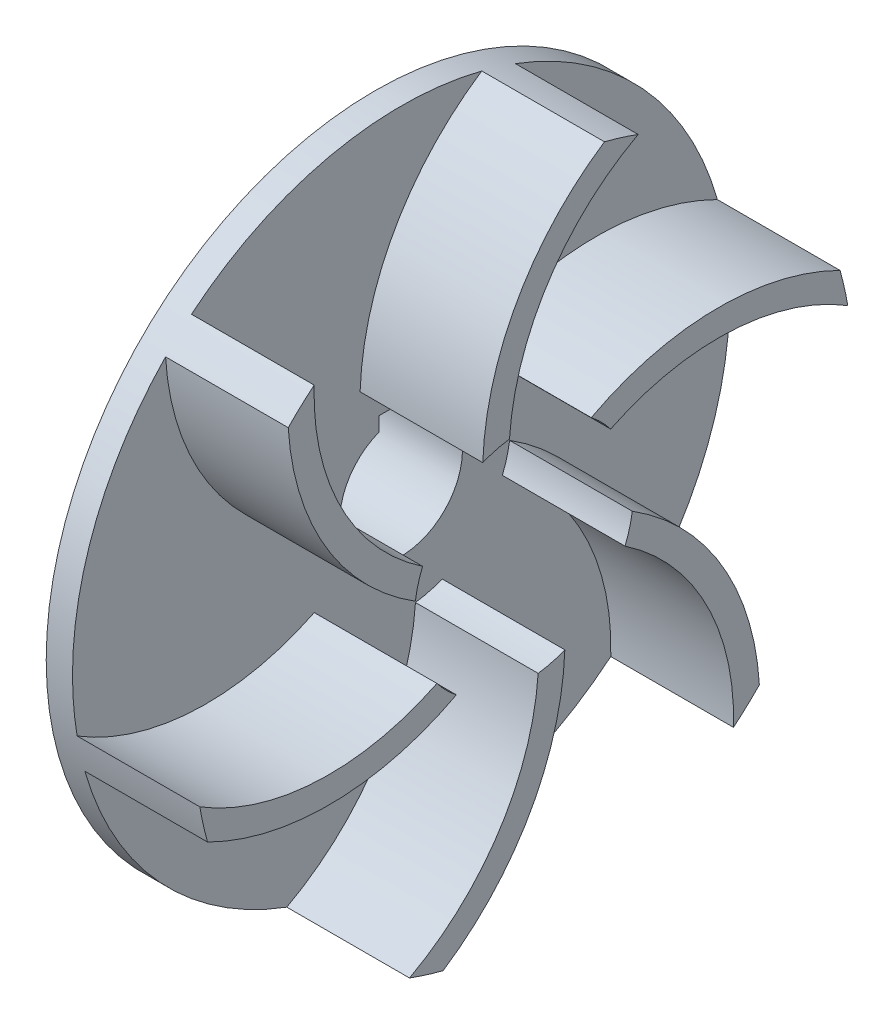
ISO-10303-21;
HEADER;
FILE_DESCRIPTION(('STEP AP214'),'2;1');
FILE_NAME('part.step','',(''),(''),'','','');
FILE_SCHEMA(('AUTOMOTIVE_DESIGN { 1 0 10303 214 1 1 1 1 }'));
ENDSEC;
DATA;
#1=APPLICATION_CONTEXT('core data for automotive mechanical design processes');
#2=APPLICATION_PROTOCOL_DEFINITION('international standard','automotive_design',2000,#1);
#3=PRODUCT_CONTEXT('',#1,'mechanical');
#4=PRODUCT('Part','Part','',(#3));
#5=PRODUCT_RELATED_PRODUCT_CATEGORY('part','',(#4));
#6=PRODUCT_DEFINITION_FORMATION('','',#4);
#7=PRODUCT_DEFINITION_CONTEXT('part definition',#1,'design');
#8=PRODUCT_DEFINITION('design','',#6,#7);
#9=PRODUCT_DEFINITION_SHAPE('','',#8);
#10=(LENGTH_UNIT() NAMED_UNIT(*) SI_UNIT(.MILLI.,.METRE.));
#11=(NAMED_UNIT(*) PLANE_ANGLE_UNIT() SI_UNIT($,.RADIAN.));
#12=(NAMED_UNIT(*) SI_UNIT($,.STERADIAN.) SOLID_ANGLE_UNIT());
#13=UNCERTAINTY_MEASURE_WITH_UNIT(LENGTH_MEASURE(1.E-05),#10,'distance_accuracy_value','');
#14=(GEOMETRIC_REPRESENTATION_CONTEXT(3) GLOBAL_UNCERTAINTY_ASSIGNED_CONTEXT((#13)) GLOBAL_UNIT_ASSIGNED_CONTEXT((#10,
#11,#12)) REPRESENTATION_CONTEXT('',''));
#15=CARTESIAN_POINT('',(0.,0.,0.));
#16=DIRECTION('',(0.,0.,1.));
#17=DIRECTION('',(1.,0.,0.));
#18=AXIS2_PLACEMENT_3D('',#15,#16,#17);
#19=CARTESIAN_POINT('',(19.,37.5,0.));
#20=DIRECTION('',(-1.,0.,0.));
#21=DIRECTION('',(0.,0.,1.));
#22=AXIS2_PLACEMENT_3D('',#19,#20,#21);
#23=PLANE('',#22);
#24=CARTESIAN_POINT('',(19.,-17.5291013565556,-22.2360825665268));
#25=DIRECTION('',(1.,0.,0.));
#26=DIRECTION('',(0.,0.,-1.));
#27=AXIS2_PLACEMENT_3D('',#24,#25,#26);
#28=CIRCLE('',#27,31.);
#29=CARTESIAN_POINT('',(19.,10.2057241564115,-36.0845284636399));
#30=VERTEX_POINT('',#29);
#31=CARTESIAN_POINT('',(19.,9.84966379316857,-7.69637077859064));
#32=VERTEX_POINT('',#31);
#33=EDGE_CURVE('E290',#30,#32,#28,.T.);
#34=ORIENTED_EDGE('',*,*,#33,.F.);
#35=CARTESIAN_POINT('',(19.,0.,0.));
#36=DIRECTION('',(-1.,0.,0.));
#37=DIRECTION('',(0.,0.,1.));
#38=AXIS2_PLACEMENT_3D('',#35,#36,#37);
#39=CIRCLE('',#38,37.5);
#40=CARTESIAN_POINT('',(19.,35.1575351750676,-13.0459848387879));
#41=VERTEX_POINT('',#40);
#42=EDGE_CURVE('E847',#41,#30,#39,.T.);
#43=ORIENTED_EDGE('',*,*,#42,.F.);
#44=CARTESIAN_POINT('',(19.,10.4924617049827,-26.2986883635528));
#45=DIRECTION('',(1.,0.,0.));
#46=DIRECTION('',(0.,0.,-1.));
#47=AXIS2_PLACEMENT_3D('',#44,#45,#46);
#48=CIRCLE('',#47,28.);
#49=CARTESIAN_POINT('',(19.,12.3923748695187,1.63677887734412));
#50=VERTEX_POINT('',#49);
#51=EDGE_CURVE('E346',#41,#50,#48,.T.);
#52=ORIENTED_EDGE('',*,*,#51,.T.);
#53=CARTESIAN_POINT('',(19.,0.,0.));
#54=DIRECTION('',(1.,0.,0.));
#55=DIRECTION('',(0.,0.,-1.));
#56=AXIS2_PLACEMENT_3D('',#53,#54,#55);
#57=CIRCLE('',#56,12.5);
#58=CARTESIAN_POINT('',(19.,11.590084507788,4.68187367432452));
#59=VERTEX_POINT('',#58);
#60=EDGE_CURVE('E354',#50,#59,#57,.T.);
#61=ORIENTED_EDGE('',*,*,#60,.T.);
#62=CARTESIAN_POINT('',(19.,10.4924617049827,-26.2986883635528));
#63=DIRECTION('',(1.,0.,0.));
#64=DIRECTION('',(0.,0.,-1.));
#65=AXIS2_PLACEMENT_3D('',#62,#63,#64);
#66=CIRCLE('',#65,31.);
#67=CARTESIAN_POINT('',(19.,36.3529804113006,-9.20384784835101));
#68=VERTEX_POINT('',#67);
#69=EDGE_CURVE('E345',#68,#59,#66,.T.);
#70=ORIENTED_EDGE('',*,*,#69,.F.);
#71=CARTESIAN_POINT('',(19.,28.8769218753108,23.9243261766596));
#72=VERTEX_POINT('',#71);
#73=EDGE_CURVE('E479',#72,#68,#39,.T.);
#74=ORIENTED_EDGE('',*,*,#73,.F.);
#75=CARTESIAN_POINT('',(19.,28.0215630615383,-4.06260579702601));
#76=DIRECTION('',(1.,0.,0.));
#77=DIRECTION('',(0.,0.,-1.));
#78=AXIS2_PLACEMENT_3D('',#75,#76,#77);
#79=CIRCLE('',#78,28.0000000000001);
#80=CARTESIAN_POINT('',(19.,4.77869534660156,11.5505008888952));
#81=VERTEX_POINT('',#80);
#82=EDGE_CURVE('E115',#72,#81,#79,.T.);
#83=ORIENTED_EDGE('',*,*,#82,.T.);
#84=CARTESIAN_POINT('',(19.,0.,0.));
#85=DIRECTION('',(1.,0.,0.));
#86=DIRECTION('',(0.,0.,-1.));
#87=AXIS2_PLACEMENT_3D('',#84,#85,#86);
#88=CIRCLE('',#87,12.5);
#89=CARTESIAN_POINT('',(19.,1.74042071461927,12.3782444529151));
#90=VERTEX_POINT('',#89);
#91=EDGE_CURVE('E318',#81,#90,#88,.T.);
#92=ORIENTED_EDGE('',*,*,#91,.T.);
#93=CARTESIAN_POINT('',(19.,28.0215630615383,-4.06260579702601));
#94=DIRECTION('',(1.,0.,0.));
#95=DIRECTION('',(0.,0.,-1.));
#96=AXIS2_PLACEMENT_3D('',#93,#94,#95);
#97=CIRCLE('',#96,31.0000000000001);
#98=CARTESIAN_POINT('',(19.,26.147256254889,26.8806806152889));
#99=VERTEX_POINT('',#98);
#100=EDGE_CURVE('E325',#99,#90,#97,.T.);
#101=ORIENTED_EDGE('',*,*,#100,.F.);
#102=CARTESIAN_POINT('',(19.,-6.28061329975611,36.9703110154476));
#103=VERTEX_POINT('',#102);
#104=EDGE_CURVE('E474',#103,#99,#39,.T.);
#105=ORIENTED_EDGE('',*,*,#104,.F.);
#106=CARTESIAN_POINT('',(19.,17.5291013565557,22.2360825665265));
#107=DIRECTION('',(1.,0.,0.));
#108=DIRECTION('',(0.,0.,-1.));
#109=AXIS2_PLACEMENT_3D('',#106,#107,#108);
#110=CIRCLE('',#109,27.9999999999998);
#111=CARTESIAN_POINT('',(19.,-7.61367952291693,9.91372201155118));
#112=VERTEX_POINT('',#111);
#113=EDGE_CURVE('E436',#103,#112,#110,.T.);
#114=ORIENTED_EDGE('',*,*,#113,.T.);
#115=CARTESIAN_POINT('',(19.,0.,0.));
#116=DIRECTION('',(1.,0.,0.));
#117=DIRECTION('',(0.,0.,-1.));
#118=AXIS2_PLACEMENT_3D('',#115,#116,#117);
#119=CIRCLE('',#118,12.5);
#120=CARTESIAN_POINT('',(19.,-9.84966379316844,7.69637077859072));
#121=VERTEX_POINT('',#120);
#122=EDGE_CURVE('E414',#112,#121,#119,.T.);
#123=ORIENTED_EDGE('',*,*,#122,.T.);
#124=CARTESIAN_POINT('',(19.,17.5291013565557,22.2360825665265));
#125=DIRECTION('',(1.,0.,0.));
#126=DIRECTION('',(0.,0.,-1.));
#127=AXIS2_PLACEMENT_3D('',#124,#125,#126);
#128=CIRCLE('',#127,30.9999999999998);
#129=CARTESIAN_POINT('',(19.,-10.2057241564109,36.0845284636401));
#130=VERTEX_POINT('',#129);
#131=EDGE_CURVE('E426',#130,#121,#128,.T.);
#132=ORIENTED_EDGE('',*,*,#131,.F.);
#133=CARTESIAN_POINT('',(19.,-35.1575351750675,13.0459848387883));
#134=VERTEX_POINT('',#133);
#135=EDGE_CURVE('E475',#134,#130,#39,.T.);
#136=ORIENTED_EDGE('',*,*,#135,.F.);
#137=CARTESIAN_POINT('',(19.,-10.4924617049824,26.2986883635528));
#138=DIRECTION('',(1.,0.,0.));
#139=DIRECTION('',(0.,0.,-1.));
#140=AXIS2_PLACEMENT_3D('',#137,#138,#139);
#141=CIRCLE('',#140,28.);
#142=CARTESIAN_POINT('',(19.,-12.3923748695188,-1.6367788773441));
#143=VERTEX_POINT('',#142);
#144=EDGE_CURVE('E408',#134,#143,#141,.T.);
#145=ORIENTED_EDGE('',*,*,#144,.T.);
#146=CARTESIAN_POINT('',(19.,0.,0.));
#147=DIRECTION('',(1.,0.,0.));
#148=DIRECTION('',(0.,0.,-1.));
#149=AXIS2_PLACEMENT_3D('',#146,#147,#148);
#150=CIRCLE('',#149,12.5);
#151=CARTESIAN_POINT('',(19.,-11.590084507788,-4.6818736743245));
#152=VERTEX_POINT('',#151);
#153=EDGE_CURVE('E406',#143,#152,#150,.T.);
#154=ORIENTED_EDGE('',*,*,#153,.T.);
#155=CARTESIAN_POINT('',(19.,-10.4924617049824,26.2986883635528));
#156=DIRECTION('',(1.,0.,0.));
#157=DIRECTION('',(0.,0.,-1.));
#158=AXIS2_PLACEMENT_3D('',#155,#156,#157);
#159=CIRCLE('',#158,31.);
#160=CARTESIAN_POINT('',(19.,-36.3529804113005,9.20384784835134));
#161=VERTEX_POINT('',#160);
#162=EDGE_CURVE('E401',#161,#152,#159,.T.);
#163=ORIENTED_EDGE('',*,*,#162,.F.);
#164=CARTESIAN_POINT('',(19.,-28.8769218753109,-23.9243261766594));
#165=VERTEX_POINT('',#164);
#166=EDGE_CURVE('E851',#165,#161,#39,.T.);
#167=ORIENTED_EDGE('',*,*,#166,.F.);
#168=CARTESIAN_POINT('',(19.,-28.0215630615381,4.06260579702616));
#169=DIRECTION('',(1.,0.,0.));
#170=DIRECTION('',(0.,0.,-1.));
#171=AXIS2_PLACEMENT_3D('',#168,#169,#170);
#172=CIRCLE('',#171,28.);
#173=CARTESIAN_POINT('',(19.,-4.77869534660156,-11.5505008888952));
#174=VERTEX_POINT('',#173);
#175=EDGE_CURVE('E380',#165,#174,#172,.T.);
#176=ORIENTED_EDGE('',*,*,#175,.T.);
#177=CARTESIAN_POINT('',(19.,0.,0.));
#178=DIRECTION('',(1.,0.,0.));
#179=DIRECTION('',(0.,0.,-1.));
#180=AXIS2_PLACEMENT_3D('',#177,#178,#179);
#181=CIRCLE('',#180,12.5);
#182=CARTESIAN_POINT('',(19.,-1.7404207146193,-12.3782444529152));
#183=VERTEX_POINT('',#182);
#184=EDGE_CURVE('E381',#174,#183,#181,.T.);
#185=ORIENTED_EDGE('',*,*,#184,.T.);
#186=CARTESIAN_POINT('',(19.,-28.0215630615381,4.06260579702616));
#187=DIRECTION('',(1.,0.,0.));
#188=DIRECTION('',(0.,0.,-1.));
#189=AXIS2_PLACEMENT_3D('',#186,#187,#188);
#190=CIRCLE('',#189,31.0000000000001);
#191=CARTESIAN_POINT('',(19.,-26.1472562548891,-26.8806806152888));
#192=VERTEX_POINT('',#191);
#193=EDGE_CURVE('E372',#192,#183,#190,.T.);
#194=ORIENTED_EDGE('',*,*,#193,.F.);
#195=CARTESIAN_POINT('',(19.,6.28061329975673,-36.9703110154475));
#196=VERTEX_POINT('',#195);
#197=EDGE_CURVE('E293',#196,#192,#39,.T.);
#198=ORIENTED_EDGE('',*,*,#197,.F.);
#199=CARTESIAN_POINT('',(19.,-17.5291013565556,-22.2360825665268));
#200=DIRECTION('',(1.,0.,0.));
#201=DIRECTION('',(0.,0.,-1.));
#202=AXIS2_PLACEMENT_3D('',#199,#200,#201);
#203=CIRCLE('',#202,28.);
#204=CARTESIAN_POINT('',(19.,7.61367952291712,-9.91372201155109));
#205=VERTEX_POINT('',#204);
#206=EDGE_CURVE('E102',#196,#205,#203,.T.);
#207=ORIENTED_EDGE('',*,*,#206,.T.);
#208=CARTESIAN_POINT('',(19.,0.,0.));
#209=DIRECTION('',(1.,0.,0.));
#210=DIRECTION('',(0.,0.,-1.));
#211=AXIS2_PLACEMENT_3D('',#208,#209,#210);
#212=CIRCLE('',#211,12.5);
#213=EDGE_CURVE('E285',#205,#32,#212,.T.);
#214=ORIENTED_EDGE('',*,*,#213,.T.);
#215=EDGE_LOOP('',(#34,#43,#52,#61,#70,#74,#83,#92,#101,#105,#114,#123,#132,#136,#145,#154,#163,
#167,#176,#185,#194,#198,#207,#214));
#216=FACE_BOUND('',#215,.T.);
#217=CARTESIAN_POINT('',(19.,0.,0.));
#218=DIRECTION('',(-1.,0.,0.));
#219=DIRECTION('',(0.,0.,1.));
#220=AXIS2_PLACEMENT_3D('',#217,#218,#219);
#221=CIRCLE('',#220,7.);
#222=CARTESIAN_POINT('',(19.,6.53834841531101,-2.5));
#223=VERTEX_POINT('',#222);
#224=CARTESIAN_POINT('',(19.,6.53834841531101,2.5));
#225=VERTEX_POINT('',#224);
#226=EDGE_CURVE('E476',#223,#225,#221,.T.);
#227=ORIENTED_EDGE('',*,*,#226,.T.);
#228=DIRECTION('',(0.,1.,0.));
#229=VECTOR('',#228,1.);
#230=CARTESIAN_POINT('',(19.,37.5,2.5));
#231=LINE('',#230,#229);
#232=CARTESIAN_POINT('',(19.,8.15,2.5));
#233=VERTEX_POINT('',#232);
#234=EDGE_CURVE('E12',#225,#233,#231,.T.);
#235=ORIENTED_EDGE('',*,*,#234,.T.);
#236=DIRECTION('',(0.,0.,-1.));
#237=VECTOR('',#236,1.);
#238=CARTESIAN_POINT('',(19.,8.15,0.));
#239=LINE('',#238,#237);
#240=CARTESIAN_POINT('',(19.,8.15,-2.5));
#241=VERTEX_POINT('',#240);
#242=EDGE_CURVE('E488',#233,#241,#239,.T.);
#243=ORIENTED_EDGE('',*,*,#242,.T.);
#244=DIRECTION('',(0.,-1.,0.));
#245=VECTOR('',#244,1.);
#246=CARTESIAN_POINT('',(19.,37.5,-2.5));
#247=LINE('',#246,#245);
#248=EDGE_CURVE('E100',#241,#223,#247,.T.);
#249=ORIENTED_EDGE('',*,*,#248,.T.);
#250=EDGE_LOOP('',(#227,#235,#243,#249));
#251=FACE_BOUND('',#250,.T.);
#252=ADVANCED_FACE('F90',(#216,#251),#23,.F.);
#253=CARTESIAN_POINT('',(-28.,0.,0.));
#254=DIRECTION('',(-1.,0.,0.));
#255=DIRECTION('',(0.,0.,1.));
#256=AXIS2_PLACEMENT_3D('',#253,#254,#255);
#257=CYLINDRICAL_SURFACE('',#256,12.5);
#258=CARTESIAN_POINT('',(0.,0.,0.));
#259=DIRECTION('',(-1.,0.,0.));
#260=DIRECTION('',(0.,0.,1.));
#261=AXIS2_PLACEMENT_3D('',#258,#259,#260);
#262=CIRCLE('',#261,12.5);
#263=CARTESIAN_POINT('',(0.,0.,12.5));
#264=VERTEX_POINT('',#263);
#265=EDGE_CURVE('E484',#264,#264,#262,.T.);
#266=ORIENTED_EDGE('',*,*,#265,.F.);
#267=EDGE_LOOP('',(#266));
#268=FACE_BOUND('',#267,.T.);
#269=CARTESIAN_POINT('',(16.,0.,0.));
#270=DIRECTION('',(-1.,0.,0.));
#271=DIRECTION('',(0.,0.,1.));
#272=AXIS2_PLACEMENT_3D('',#269,#270,#271);
#273=CIRCLE('',#272,12.5);
#274=CARTESIAN_POINT('',(16.,0.,12.5));
#275=VERTEX_POINT('',#274);
#276=EDGE_CURVE('E469',#275,#275,#273,.T.);
#277=ORIENTED_EDGE('',*,*,#276,.T.);
#278=EDGE_LOOP('',(#277));
#279=FACE_BOUND('',#278,.T.);
#280=ADVANCED_FACE('F93',(#268,#279),#257,.T.);
#281=CARTESIAN_POINT('',(0.,12.5,0.));
#282=DIRECTION('',(1.,0.,0.));
#283=DIRECTION('',(0.,0.,-1.));
#284=AXIS2_PLACEMENT_3D('',#281,#282,#283);
#285=PLANE('',#284);
#286=DIRECTION('',(0.,0.,-1.));
#287=VECTOR('',#286,1.);
#288=CARTESIAN_POINT('',(0.,8.15,-2.5));
#289=LINE('',#288,#287);
#290=CARTESIAN_POINT('',(0.,8.15,2.5));
#291=VERTEX_POINT('',#290);
#292=CARTESIAN_POINT('',(0.,8.15,-2.5));
#293=VERTEX_POINT('',#292);
#294=EDGE_CURVE('E452',#291,#293,#289,.T.);
#295=ORIENTED_EDGE('',*,*,#294,.F.);
#296=DIRECTION('',(0.,1.,0.));
#297=VECTOR('',#296,1.);
#298=CARTESIAN_POINT('',(0.,8.15,2.5));
#299=LINE('',#298,#297);
#300=CARTESIAN_POINT('',(0.,6.53834841531101,2.5));
#301=VERTEX_POINT('',#300);
#302=EDGE_CURVE('E446',#301,#291,#299,.T.);
#303=ORIENTED_EDGE('',*,*,#302,.F.);
#304=CARTESIAN_POINT('',(0.,0.,0.));
#305=DIRECTION('',(-1.,0.,0.));
#306=DIRECTION('',(0.,0.,1.));
#307=AXIS2_PLACEMENT_3D('',#304,#305,#306);
#308=CIRCLE('',#307,7.);
#309=CARTESIAN_POINT('',(0.,6.53834841531101,-2.5));
#310=VERTEX_POINT('',#309);
#311=EDGE_CURVE('E485',#310,#301,#308,.T.);
#312=ORIENTED_EDGE('',*,*,#311,.F.);
#313=DIRECTION('',(0.,-1.,0.));
#314=VECTOR('',#313,1.);
#315=CARTESIAN_POINT('',(0.,8.15,-2.5));
#316=LINE('',#315,#314);
#317=EDGE_CURVE('E455',#293,#310,#316,.T.);
#318=ORIENTED_EDGE('',*,*,#317,.F.);
#319=EDGE_LOOP('',(#295,#303,#312,#318));
#320=FACE_BOUND('',#319,.T.);
#321=ORIENTED_EDGE('',*,*,#265,.T.);
#322=EDGE_LOOP('',(#321));
#323=FACE_BOUND('',#322,.T.);
#324=ADVANCED_FACE('F502',(#320,#323),#285,.F.);
#325=CARTESIAN_POINT('',(-28.,0.,0.));
#326=DIRECTION('',(-1.,0.,0.));
#327=DIRECTION('',(0.,0.,1.));
#328=AXIS2_PLACEMENT_3D('',#325,#326,#327);
#329=CYLINDRICAL_SURFACE('',#328,7.);
#330=ORIENTED_EDGE('',*,*,#311,.T.);
#331=DIRECTION('',(-1.,0.,0.));
#332=VECTOR('',#331,1.);
#333=CARTESIAN_POINT('',(-28.,6.53834841531101,2.5));
#334=LINE('',#333,#332);
#335=EDGE_CURVE('E461',#301,#225,#334,.F.);
#336=ORIENTED_EDGE('',*,*,#335,.T.);
#337=ORIENTED_EDGE('',*,*,#226,.F.);
#338=DIRECTION('',(-1.,0.,0.));
#339=VECTOR('',#338,1.);
#340=CARTESIAN_POINT('',(-28.,6.53834841531101,-2.5));
#341=LINE('',#340,#339);
#342=EDGE_CURVE('E458',#223,#310,#341,.T.);
#343=ORIENTED_EDGE('',*,*,#342,.T.);
#344=EDGE_LOOP('',(#330,#336,#337,#343));
#345=FACE_BOUND('',#344,.T.);
#346=ADVANCED_FACE('F494',(#345),#329,.F.);
#347=CARTESIAN_POINT('',(-28.,0.,0.));
#348=DIRECTION('',(-1.,0.,0.));
#349=DIRECTION('',(0.,0.,1.));
#350=AXIS2_PLACEMENT_3D('',#347,#348,#349);
#351=CYLINDRICAL_SURFACE('',#350,37.5);
#352=CARTESIAN_POINT('',(16.,0.,0.));
#353=DIRECTION('',(-1.,0.,0.));
#354=DIRECTION('',(0.,0.,1.));
#355=AXIS2_PLACEMENT_3D('',#352,#353,#354);
#356=CIRCLE('',#355,37.5);
#357=CARTESIAN_POINT('',(16.,0.,37.5));
#358=VERTEX_POINT('',#357);
#359=EDGE_CURVE('E473',#358,#358,#356,.T.);
#360=ORIENTED_EDGE('',*,*,#359,.F.);
#361=EDGE_LOOP('',(#360));
#362=FACE_BOUND('',#361,.T.);
#363=ORIENTED_EDGE('',*,*,#104,.T.);
#364=DIRECTION('',(-1.,0.,0.));
#365=VECTOR('',#364,1.);
#366=CARTESIAN_POINT('',(33.,26.147256254889,26.8806806152889));
#367=LINE('',#366,#365);
#368=CARTESIAN_POINT('',(33.,26.147256254889,26.8806806152889));
#369=VERTEX_POINT('',#368);
#370=EDGE_CURVE('E303',#369,#99,#367,.T.);
#371=ORIENTED_EDGE('',*,*,#370,.F.);
#372=CARTESIAN_POINT('',(33.,0.,0.));
#373=DIRECTION('',(1.,0.,0.));
#374=DIRECTION('',(0.,0.,-1.));
#375=AXIS2_PLACEMENT_3D('',#372,#373,#374);
#376=CIRCLE('',#375,37.5);
#377=CARTESIAN_POINT('',(33.,28.8769218753108,23.9243261766596));
#378=VERTEX_POINT('',#377);
#379=EDGE_CURVE('E317',#378,#369,#376,.T.);
#380=ORIENTED_EDGE('',*,*,#379,.F.);
#381=DIRECTION('',(-1.,0.,0.));
#382=VECTOR('',#381,1.);
#383=CARTESIAN_POINT('',(33.,28.8769218753108,23.9243261766596));
#384=LINE('',#383,#382);
#385=EDGE_CURVE('E314',#378,#72,#384,.T.);
#386=ORIENTED_EDGE('',*,*,#385,.T.);
#387=ORIENTED_EDGE('',*,*,#73,.T.);
#388=DIRECTION('',(-1.,0.,0.));
#389=VECTOR('',#388,1.);
#390=CARTESIAN_POINT('',(33.,36.3529804113006,-9.20384784835101));
#391=LINE('',#390,#389);
#392=CARTESIAN_POINT('',(33.,36.3529804113006,-9.20384784835101));
#393=VERTEX_POINT('',#392);
#394=EDGE_CURVE('E340',#393,#68,#391,.T.);
#395=ORIENTED_EDGE('',*,*,#394,.F.);
#396=CARTESIAN_POINT('',(33.,0.,0.));
#397=DIRECTION('',(1.,0.,0.));
#398=DIRECTION('',(0.,0.,-1.));
#399=AXIS2_PLACEMENT_3D('',#396,#397,#398);
#400=CIRCLE('',#399,37.5);
#401=CARTESIAN_POINT('',(33.,35.1575351750676,-13.0459848387879));
#402=VERTEX_POINT('',#401);
#403=EDGE_CURVE('E357',#402,#393,#400,.T.);
#404=ORIENTED_EDGE('',*,*,#403,.F.);
#405=DIRECTION('',(-1.,0.,0.));
#406=VECTOR('',#405,1.);
#407=CARTESIAN_POINT('',(33.,35.1575351750676,-13.0459848387879));
#408=LINE('',#407,#406);
#409=EDGE_CURVE('E338',#402,#41,#408,.T.);
#410=ORIENTED_EDGE('',*,*,#409,.T.);
#411=ORIENTED_EDGE('',*,*,#42,.T.);
#412=DIRECTION('',(-1.,0.,0.));
#413=VECTOR('',#412,1.);
#414=CARTESIAN_POINT('',(33.,10.2057241564115,-36.0845284636399));
#415=LINE('',#414,#413);
#416=CARTESIAN_POINT('',(33.,10.2057241564115,-36.0845284636399));
#417=VERTEX_POINT('',#416);
#418=EDGE_CURVE('E848',#417,#30,#415,.T.);
#419=ORIENTED_EDGE('',*,*,#418,.F.);
#420=CARTESIAN_POINT('',(33.,0.,0.));
#421=DIRECTION('',(1.,0.,0.));
#422=DIRECTION('',(0.,0.,-1.));
#423=AXIS2_PLACEMENT_3D('',#420,#421,#422);
#424=CIRCLE('',#423,37.5);
#425=CARTESIAN_POINT('',(33.,6.28061329975673,-36.9703110154475));
#426=VERTEX_POINT('',#425);
#427=EDGE_CURVE('E298',#426,#417,#424,.T.);
#428=ORIENTED_EDGE('',*,*,#427,.F.);
#429=DIRECTION('',(-1.,0.,0.));
#430=VECTOR('',#429,1.);
#431=CARTESIAN_POINT('',(33.,6.28061329975673,-36.9703110154475));
#432=LINE('',#431,#430);
#433=EDGE_CURVE('E278',#426,#196,#432,.T.);
#434=ORIENTED_EDGE('',*,*,#433,.T.);
#435=ORIENTED_EDGE('',*,*,#197,.T.);
#436=DIRECTION('',(-1.,0.,0.));
#437=VECTOR('',#436,1.);
#438=CARTESIAN_POINT('',(33.,-26.1472562548891,-26.8806806152888));
#439=LINE('',#438,#437);
#440=CARTESIAN_POINT('',(33.,-26.1472562548891,-26.8806806152888));
#441=VERTEX_POINT('',#440);
#442=EDGE_CURVE('E366',#441,#192,#439,.T.);
#443=ORIENTED_EDGE('',*,*,#442,.F.);
#444=CARTESIAN_POINT('',(33.,0.,0.));
#445=DIRECTION('',(1.,0.,0.));
#446=DIRECTION('',(0.,0.,-1.));
#447=AXIS2_PLACEMENT_3D('',#444,#445,#446);
#448=CIRCLE('',#447,37.5);
#449=CARTESIAN_POINT('',(33.,-28.8769218753109,-23.9243261766594));
#450=VERTEX_POINT('',#449);
#451=EDGE_CURVE('E387',#450,#441,#448,.T.);
#452=ORIENTED_EDGE('',*,*,#451,.F.);
#453=DIRECTION('',(-1.,0.,0.));
#454=VECTOR('',#453,1.);
#455=CARTESIAN_POINT('',(33.,-28.8769218753109,-23.9243261766594));
#456=LINE('',#455,#454);
#457=EDGE_CURVE('E364',#450,#165,#456,.T.);
#458=ORIENTED_EDGE('',*,*,#457,.T.);
#459=ORIENTED_EDGE('',*,*,#166,.T.);
#460=DIRECTION('',(-1.,0.,0.));
#461=VECTOR('',#460,1.);
#462=CARTESIAN_POINT('',(33.,-36.3529804113005,9.20384784835134));
#463=LINE('',#462,#461);
#464=CARTESIAN_POINT('',(33.,-36.3529804113005,9.20384784835134));
#465=VERTEX_POINT('',#464);
#466=EDGE_CURVE('E397',#465,#161,#463,.T.);
#467=ORIENTED_EDGE('',*,*,#466,.F.);
#468=CARTESIAN_POINT('',(33.,0.,0.));
#469=DIRECTION('',(1.,0.,0.));
#470=DIRECTION('',(0.,0.,-1.));
#471=AXIS2_PLACEMENT_3D('',#468,#469,#470);
#472=CIRCLE('',#471,37.5);
#473=CARTESIAN_POINT('',(33.,-35.1575351750675,13.0459848387883));
#474=VERTEX_POINT('',#473);
#475=EDGE_CURVE('E415',#474,#465,#472,.T.);
#476=ORIENTED_EDGE('',*,*,#475,.F.);
#477=DIRECTION('',(-1.,0.,0.));
#478=VECTOR('',#477,1.);
#479=CARTESIAN_POINT('',(33.,-35.1575351750675,13.0459848387883));
#480=LINE('',#479,#478);
#481=EDGE_CURVE('E395',#474,#134,#480,.T.);
#482=ORIENTED_EDGE('',*,*,#481,.T.);
#483=ORIENTED_EDGE('',*,*,#135,.T.);
#484=DIRECTION('',(-1.,0.,0.));
#485=VECTOR('',#484,1.);
#486=CARTESIAN_POINT('',(33.,-10.2057241564109,36.0845284636401));
#487=LINE('',#486,#485);
#488=CARTESIAN_POINT('',(33.,-10.2057241564109,36.0845284636401));
#489=VERTEX_POINT('',#488);
#490=EDGE_CURVE('E445',#489,#130,#487,.T.);
#491=ORIENTED_EDGE('',*,*,#490,.F.);
#492=CARTESIAN_POINT('',(33.,0.,0.));
#493=DIRECTION('',(1.,0.,0.));
#494=DIRECTION('',(0.,0.,-1.));
#495=AXIS2_PLACEMENT_3D('',#492,#493,#494);
#496=CIRCLE('',#495,37.5);
#497=CARTESIAN_POINT('',(33.,-6.28061329975611,36.9703110154476));
#498=VERTEX_POINT('',#497);
#499=EDGE_CURVE('E427',#498,#489,#496,.T.);
#500=ORIENTED_EDGE('',*,*,#499,.F.);
#501=DIRECTION('',(-1.,0.,0.));
#502=VECTOR('',#501,1.);
#503=CARTESIAN_POINT('',(33.,-6.28061329975611,36.9703110154476));
#504=LINE('',#503,#502);
#505=EDGE_CURVE('E443',#498,#103,#504,.T.);
#506=ORIENTED_EDGE('',*,*,#505,.T.);
#507=EDGE_LOOP('',(#363,#371,#380,#386,#387,#395,#404,#410,#411,#419,#428,#434,#435,#443,#452,
#458,#459,#467,#476,#482,#483,#491,#500,#506));
#508=FACE_BOUND('',#507,.T.);
#509=ADVANCED_FACE('F530',(#362,#508),#351,.T.);
#510=CARTESIAN_POINT('',(16.,12.5,0.));
#511=DIRECTION('',(1.,0.,0.));
#512=DIRECTION('',(0.,0.,-1.));
#513=AXIS2_PLACEMENT_3D('',#510,#511,#512);
#514=PLANE('',#513);
#515=ORIENTED_EDGE('',*,*,#276,.F.);
#516=EDGE_LOOP('',(#515));
#517=FACE_BOUND('',#516,.T.);
#518=ORIENTED_EDGE('',*,*,#359,.T.);
#519=EDGE_LOOP('',(#518));
#520=FACE_BOUND('',#519,.T.);
#521=ADVANCED_FACE('F519',(#517,#520),#514,.F.);
#522=CARTESIAN_POINT('',(30.,8.15,2.5));
#523=DIRECTION('',(0.,0.,1.));
#524=DIRECTION('',(1.,0.,0.));
#525=AXIS2_PLACEMENT_3D('',#522,#523,#524);
#526=PLANE('',#525);
#527=ORIENTED_EDGE('',*,*,#302,.T.);
#528=DIRECTION('',(-1.,0.,0.));
#529=VECTOR('',#528,1.);
#530=CARTESIAN_POINT('',(30.,8.15,2.5));
#531=LINE('',#530,#529);
#532=EDGE_CURVE('E460',#233,#291,#531,.T.);
#533=ORIENTED_EDGE('',*,*,#532,.F.);
#534=ORIENTED_EDGE('',*,*,#234,.F.);
#535=ORIENTED_EDGE('',*,*,#335,.F.);
#536=EDGE_LOOP('',(#527,#533,#534,#535));
#537=FACE_BOUND('',#536,.T.);
#538=ADVANCED_FACE('F496',(#537),#526,.F.);
#539=CARTESIAN_POINT('',(30.,8.15,-2.5));
#540=DIRECTION('',(0.,0.,-1.));
#541=DIRECTION('',(-1.,0.,0.));
#542=AXIS2_PLACEMENT_3D('',#539,#540,#541);
#543=PLANE('',#542);
#544=ORIENTED_EDGE('',*,*,#248,.F.);
#545=DIRECTION('',(-1.,0.,0.));
#546=VECTOR('',#545,1.);
#547=CARTESIAN_POINT('',(30.,8.15,-2.5));
#548=LINE('',#547,#546);
#549=EDGE_CURVE('E456',#241,#293,#548,.T.);
#550=ORIENTED_EDGE('',*,*,#549,.T.);
#551=ORIENTED_EDGE('',*,*,#317,.T.);
#552=ORIENTED_EDGE('',*,*,#342,.F.);
#553=EDGE_LOOP('',(#544,#550,#551,#552));
#554=FACE_BOUND('',#553,.T.);
#555=ADVANCED_FACE('F509',(#554),#543,.F.);
#556=CARTESIAN_POINT('',(30.,8.15,-2.5));
#557=DIRECTION('',(0.,1.,0.));
#558=DIRECTION('',(0.,0.,1.));
#559=AXIS2_PLACEMENT_3D('',#556,#557,#558);
#560=PLANE('',#559);
#561=ORIENTED_EDGE('',*,*,#532,.T.);
#562=ORIENTED_EDGE('',*,*,#294,.T.);
#563=ORIENTED_EDGE('',*,*,#549,.F.);
#564=ORIENTED_EDGE('',*,*,#242,.F.);
#565=EDGE_LOOP('',(#561,#562,#563,#564));
#566=FACE_BOUND('',#565,.T.);
#567=ADVANCED_FACE('F507',(#566),#560,.F.);
#568=CARTESIAN_POINT('',(33.,0.,0.));
#569=DIRECTION('',(-1.,0.,0.));
#570=DIRECTION('',(0.,0.,1.));
#571=AXIS2_PLACEMENT_3D('',#568,#569,#570);
#572=CYLINDRICAL_SURFACE('',#571,12.5);
#573=ORIENTED_EDGE('',*,*,#122,.F.);
#574=DIRECTION('',(-1.,0.,0.));
#575=VECTOR('',#574,1.);
#576=CARTESIAN_POINT('',(33.,-7.61367952291693,9.91372201155118));
#577=LINE('',#576,#575);
#578=CARTESIAN_POINT('',(33.,-7.61367952291693,9.91372201155118));
#579=VERTEX_POINT('',#578);
#580=EDGE_CURVE('E449',#579,#112,#577,.T.);
#581=ORIENTED_EDGE('',*,*,#580,.F.);
#582=CARTESIAN_POINT('',(33.,0.,0.));
#583=DIRECTION('',(1.,0.,0.));
#584=DIRECTION('',(0.,0.,-1.));
#585=AXIS2_PLACEMENT_3D('',#582,#583,#584);
#586=CIRCLE('',#585,12.5);
#587=CARTESIAN_POINT('',(33.,-9.84966379316844,7.69637077859072));
#588=VERTEX_POINT('',#587);
#589=EDGE_CURVE('E425',#579,#588,#586,.T.);
#590=ORIENTED_EDGE('',*,*,#589,.T.);
#591=DIRECTION('',(-1.,0.,0.));
#592=VECTOR('',#591,1.);
#593=CARTESIAN_POINT('',(33.,-9.84966379316844,7.69637077859072));
#594=LINE('',#593,#592);
#595=EDGE_CURVE('E433',#588,#121,#594,.T.);
#596=ORIENTED_EDGE('',*,*,#595,.T.);
#597=EDGE_LOOP('',(#573,#581,#590,#596));
#598=FACE_BOUND('',#597,.T.);
#599=ADVANCED_FACE('F513',(#598),#572,.F.);
#600=CARTESIAN_POINT('',(33.,17.5291013565557,22.2360825665265));
#601=DIRECTION('',(-1.,0.,0.));
#602=DIRECTION('',(0.,0.,1.));
#603=AXIS2_PLACEMENT_3D('',#600,#601,#602);
#604=CYLINDRICAL_SURFACE('',#603,27.9999999999998);
#605=ORIENTED_EDGE('',*,*,#113,.F.);
#606=ORIENTED_EDGE('',*,*,#505,.F.);
#607=CARTESIAN_POINT('',(33.,17.5291013565557,22.2360825665265));
#608=DIRECTION('',(1.,0.,0.));
#609=DIRECTION('',(0.,0.,-1.));
#610=AXIS2_PLACEMENT_3D('',#607,#608,#609);
#611=CIRCLE('',#610,27.9999999999998);
#612=EDGE_CURVE('E422',#498,#579,#611,.T.);
#613=ORIENTED_EDGE('',*,*,#612,.T.);
#614=ORIENTED_EDGE('',*,*,#580,.T.);
#615=EDGE_LOOP('',(#605,#606,#613,#614));
#616=FACE_BOUND('',#615,.T.);
#617=ADVANCED_FACE('F614',(#616),#604,.F.);
#618=CARTESIAN_POINT('',(33.,17.5291013565557,22.2360825665265));
#619=DIRECTION('',(-1.,0.,0.));
#620=DIRECTION('',(0.,0.,1.));
#621=AXIS2_PLACEMENT_3D('',#618,#619,#620);
#622=CYLINDRICAL_SURFACE('',#621,30.9999999999998);
#623=ORIENTED_EDGE('',*,*,#131,.T.);
#624=ORIENTED_EDGE('',*,*,#595,.F.);
#625=CARTESIAN_POINT('',(33.,17.5291013565557,22.2360825665265));
#626=DIRECTION('',(1.,0.,0.));
#627=DIRECTION('',(0.,0.,-1.));
#628=AXIS2_PLACEMENT_3D('',#625,#626,#627);
#629=CIRCLE('',#628,30.9999999999998);
#630=EDGE_CURVE('E431',#489,#588,#629,.T.);
#631=ORIENTED_EDGE('',*,*,#630,.F.);
#632=ORIENTED_EDGE('',*,*,#490,.T.);
#633=EDGE_LOOP('',(#623,#624,#631,#632));
#634=FACE_BOUND('',#633,.T.);
#635=ADVANCED_FACE('F622',(#634),#622,.T.);
#636=CARTESIAN_POINT('',(33.,0.,0.));
#637=DIRECTION('',(1.,0.,0.));
#638=DIRECTION('',(0.,0.,-1.));
#639=AXIS2_PLACEMENT_3D('',#636,#637,#638);
#640=PLANE('',#639);
#641=ORIENTED_EDGE('',*,*,#589,.F.);
#642=ORIENTED_EDGE('',*,*,#612,.F.);
#643=ORIENTED_EDGE('',*,*,#499,.T.);
#644=ORIENTED_EDGE('',*,*,#630,.T.);
#645=EDGE_LOOP('',(#641,#642,#643,#644));
#646=FACE_BOUND('',#645,.T.);
#647=ADVANCED_FACE('F631',(#646),#640,.T.);
#648=CARTESIAN_POINT('',(33.,0.,0.));
#649=DIRECTION('',(-1.,0.,0.));
#650=DIRECTION('',(0.,0.,1.));
#651=AXIS2_PLACEMENT_3D('',#648,#649,#650);
#652=CYLINDRICAL_SURFACE('',#651,12.5);
#653=ORIENTED_EDGE('',*,*,#153,.F.);
#654=DIRECTION('',(-1.,0.,0.));
#655=VECTOR('',#654,1.);
#656=CARTESIAN_POINT('',(33.,-12.3923748695188,-1.6367788773441));
#657=LINE('',#656,#655);
#658=CARTESIAN_POINT('',(33.,-12.3923748695188,-1.6367788773441));
#659=VERTEX_POINT('',#658);
#660=EDGE_CURVE('E383',#659,#143,#657,.T.);
#661=ORIENTED_EDGE('',*,*,#660,.F.);
#662=CARTESIAN_POINT('',(33.,0.,0.));
#663=DIRECTION('',(1.,0.,0.));
#664=DIRECTION('',(0.,0.,-1.));
#665=AXIS2_PLACEMENT_3D('',#662,#663,#664);
#666=CIRCLE('',#665,12.5);
#667=CARTESIAN_POINT('',(33.,-11.590084507788,-4.6818736743245));
#668=VERTEX_POINT('',#667);
#669=EDGE_CURVE('E409',#659,#668,#666,.T.);
#670=ORIENTED_EDGE('',*,*,#669,.T.);
#671=DIRECTION('',(-1.,0.,0.));
#672=VECTOR('',#671,1.);
#673=CARTESIAN_POINT('',(33.,-11.590084507788,-4.6818736743245));
#674=LINE('',#673,#672);
#675=EDGE_CURVE('E400',#668,#152,#674,.T.);
#676=ORIENTED_EDGE('',*,*,#675,.T.);
#677=EDGE_LOOP('',(#653,#661,#670,#676));
#678=FACE_BOUND('',#677,.T.);
#679=ADVANCED_FACE('F643',(#678),#652,.F.);
#680=CARTESIAN_POINT('',(33.,-10.4924617049824,26.2986883635528));
#681=DIRECTION('',(-1.,0.,0.));
#682=DIRECTION('',(0.,0.,1.));
#683=AXIS2_PLACEMENT_3D('',#680,#681,#682);
#684=CYLINDRICAL_SURFACE('',#683,28.);
#685=ORIENTED_EDGE('',*,*,#144,.F.);
#686=ORIENTED_EDGE('',*,*,#481,.F.);
#687=CARTESIAN_POINT('',(33.,-10.4924617049824,26.2986883635528));
#688=DIRECTION('',(1.,0.,0.));
#689=DIRECTION('',(0.,0.,-1.));
#690=AXIS2_PLACEMENT_3D('',#687,#688,#689);
#691=CIRCLE('',#690,28.);
#692=EDGE_CURVE('E417',#474,#659,#691,.T.);
#693=ORIENTED_EDGE('',*,*,#692,.T.);
#694=ORIENTED_EDGE('',*,*,#660,.T.);
#695=EDGE_LOOP('',(#685,#686,#693,#694));
#696=FACE_BOUND('',#695,.T.);
#697=ADVANCED_FACE('F651',(#696),#684,.F.);
#698=CARTESIAN_POINT('',(33.,-10.4924617049824,26.2986883635528));
#699=DIRECTION('',(-1.,0.,0.));
#700=DIRECTION('',(0.,0.,1.));
#701=AXIS2_PLACEMENT_3D('',#698,#699,#700);
#702=CYLINDRICAL_SURFACE('',#701,31.);
#703=ORIENTED_EDGE('',*,*,#162,.T.);
#704=ORIENTED_EDGE('',*,*,#675,.F.);
#705=CARTESIAN_POINT('',(33.,-10.4924617049824,26.2986883635528));
#706=DIRECTION('',(1.,0.,0.));
#707=DIRECTION('',(0.,0.,-1.));
#708=AXIS2_PLACEMENT_3D('',#705,#706,#707);
#709=CIRCLE('',#708,31.);
#710=EDGE_CURVE('E405',#465,#668,#709,.T.);
#711=ORIENTED_EDGE('',*,*,#710,.F.);
#712=ORIENTED_EDGE('',*,*,#466,.T.);
#713=EDGE_LOOP('',(#703,#704,#711,#712));
#714=FACE_BOUND('',#713,.T.);
#715=ADVANCED_FACE('F662',(#714),#702,.T.);
#716=CARTESIAN_POINT('',(33.,0.,0.));
#717=DIRECTION('',(1.,0.,0.));
#718=DIRECTION('',(0.,0.,-1.));
#719=AXIS2_PLACEMENT_3D('',#716,#717,#718);
#720=PLANE('',#719);
#721=ORIENTED_EDGE('',*,*,#669,.F.);
#722=ORIENTED_EDGE('',*,*,#692,.F.);
#723=ORIENTED_EDGE('',*,*,#475,.T.);
#724=ORIENTED_EDGE('',*,*,#710,.T.);
#725=EDGE_LOOP('',(#721,#722,#723,#724));
#726=FACE_BOUND('',#725,.T.);
#727=ADVANCED_FACE('F671',(#726),#720,.T.);
#728=CARTESIAN_POINT('',(33.,0.,0.));
#729=DIRECTION('',(-1.,0.,0.));
#730=DIRECTION('',(0.,0.,1.));
#731=AXIS2_PLACEMENT_3D('',#728,#729,#730);
#732=CYLINDRICAL_SURFACE('',#731,12.5);
#733=ORIENTED_EDGE('',*,*,#184,.F.);
#734=DIRECTION('',(-1.,0.,0.));
#735=VECTOR('',#734,1.);
#736=CARTESIAN_POINT('',(33.,-4.77869534660156,-11.5505008888952));
#737=LINE('',#736,#735);
#738=CARTESIAN_POINT('',(33.,-4.77869534660156,-11.5505008888952));
#739=VERTEX_POINT('',#738);
#740=EDGE_CURVE('E351',#739,#174,#737,.T.);
#741=ORIENTED_EDGE('',*,*,#740,.F.);
#742=CARTESIAN_POINT('',(33.,0.,0.));
#743=DIRECTION('',(1.,0.,0.));
#744=DIRECTION('',(0.,0.,-1.));
#745=AXIS2_PLACEMENT_3D('',#742,#743,#744);
#746=CIRCLE('',#745,12.5);
#747=CARTESIAN_POINT('',(33.,-1.7404207146193,-12.3782444529152));
#748=VERTEX_POINT('',#747);
#749=EDGE_CURVE('E378',#739,#748,#746,.T.);
#750=ORIENTED_EDGE('',*,*,#749,.T.);
#751=DIRECTION('',(-1.,0.,0.));
#752=VECTOR('',#751,1.);
#753=CARTESIAN_POINT('',(33.,-1.7404207146193,-12.3782444529152));
#754=LINE('',#753,#752);
#755=EDGE_CURVE('E371',#748,#183,#754,.T.);
#756=ORIENTED_EDGE('',*,*,#755,.T.);
#757=EDGE_LOOP('',(#733,#741,#750,#756));
#758=FACE_BOUND('',#757,.T.);
#759=ADVANCED_FACE('F683',(#758),#732,.F.);
#760=CARTESIAN_POINT('',(33.,-28.0215630615381,4.06260579702616));
#761=DIRECTION('',(-1.,0.,0.));
#762=DIRECTION('',(0.,0.,1.));
#763=AXIS2_PLACEMENT_3D('',#760,#761,#762);
#764=CYLINDRICAL_SURFACE('',#763,28.);
#765=ORIENTED_EDGE('',*,*,#175,.F.);
#766=ORIENTED_EDGE('',*,*,#457,.F.);
#767=CARTESIAN_POINT('',(33.,-28.0215630615381,4.06260579702616));
#768=DIRECTION('',(1.,0.,0.));
#769=DIRECTION('',(0.,0.,-1.));
#770=AXIS2_PLACEMENT_3D('',#767,#768,#769);
#771=CIRCLE('',#770,28.);
#772=EDGE_CURVE('E389',#450,#739,#771,.T.);
#773=ORIENTED_EDGE('',*,*,#772,.T.);
#774=ORIENTED_EDGE('',*,*,#740,.T.);
#775=EDGE_LOOP('',(#765,#766,#773,#774));
#776=FACE_BOUND('',#775,.T.);
#777=ADVANCED_FACE('F695',(#776),#764,.F.);
#778=CARTESIAN_POINT('',(33.,-28.0215630615381,4.06260579702616));
#779=DIRECTION('',(-1.,0.,0.));
#780=DIRECTION('',(0.,0.,1.));
#781=AXIS2_PLACEMENT_3D('',#778,#779,#780);
#782=CYLINDRICAL_SURFACE('',#781,31.0000000000001);
#783=ORIENTED_EDGE('',*,*,#193,.T.);
#784=ORIENTED_EDGE('',*,*,#755,.F.);
#785=CARTESIAN_POINT('',(33.,-28.0215630615381,4.06260579702616));
#786=DIRECTION('',(1.,0.,0.));
#787=DIRECTION('',(0.,0.,-1.));
#788=AXIS2_PLACEMENT_3D('',#785,#786,#787);
#789=CIRCLE('',#788,31.0000000000001);
#790=EDGE_CURVE('E373',#441,#748,#789,.T.);
#791=ORIENTED_EDGE('',*,*,#790,.F.);
#792=ORIENTED_EDGE('',*,*,#442,.T.);
#793=EDGE_LOOP('',(#783,#784,#791,#792));
#794=FACE_BOUND('',#793,.T.);
#795=ADVANCED_FACE('F702',(#794),#782,.T.);
#796=CARTESIAN_POINT('',(33.,0.,0.));
#797=DIRECTION('',(1.,0.,0.));
#798=DIRECTION('',(0.,0.,-1.));
#799=AXIS2_PLACEMENT_3D('',#796,#797,#798);
#800=PLANE('',#799);
#801=ORIENTED_EDGE('',*,*,#749,.F.);
#802=ORIENTED_EDGE('',*,*,#772,.F.);
#803=ORIENTED_EDGE('',*,*,#451,.T.);
#804=ORIENTED_EDGE('',*,*,#790,.T.);
#805=EDGE_LOOP('',(#801,#802,#803,#804));
#806=FACE_BOUND('',#805,.T.);
#807=ADVANCED_FACE('F713',(#806),#800,.T.);
#808=CARTESIAN_POINT('',(33.,0.,0.));
#809=DIRECTION('',(-1.,0.,0.));
#810=DIRECTION('',(0.,0.,1.));
#811=AXIS2_PLACEMENT_3D('',#808,#809,#810);
#812=CYLINDRICAL_SURFACE('',#811,12.5);
#813=ORIENTED_EDGE('',*,*,#60,.F.);
#814=DIRECTION('',(-1.,0.,0.));
#815=VECTOR('',#814,1.);
#816=CARTESIAN_POINT('',(33.,12.3923748695187,1.63677887734412));
#817=LINE('',#816,#815);
#818=CARTESIAN_POINT('',(33.,12.3923748695187,1.63677887734412));
#819=VERTEX_POINT('',#818);
#820=EDGE_CURVE('E324',#819,#50,#817,.T.);
#821=ORIENTED_EDGE('',*,*,#820,.F.);
#822=CARTESIAN_POINT('',(33.,0.,0.));
#823=DIRECTION('',(1.,0.,0.));
#824=DIRECTION('',(0.,0.,-1.));
#825=AXIS2_PLACEMENT_3D('',#822,#823,#824);
#826=CIRCLE('',#825,12.5);
#827=CARTESIAN_POINT('',(33.,11.590084507788,4.68187367432452));
#828=VERTEX_POINT('',#827);
#829=EDGE_CURVE('E349',#819,#828,#826,.T.);
#830=ORIENTED_EDGE('',*,*,#829,.T.);
#831=DIRECTION('',(-1.,0.,0.));
#832=VECTOR('',#831,1.);
#833=CARTESIAN_POINT('',(33.,11.590084507788,4.68187367432452));
#834=LINE('',#833,#832);
#835=EDGE_CURVE('E342',#828,#59,#834,.T.);
#836=ORIENTED_EDGE('',*,*,#835,.T.);
#837=EDGE_LOOP('',(#813,#821,#830,#836));
#838=FACE_BOUND('',#837,.T.);
#839=ADVANCED_FACE('F725',(#838),#812,.F.);
#840=CARTESIAN_POINT('',(33.,10.4924617049827,-26.2986883635528));
#841=DIRECTION('',(-1.,0.,0.));
#842=DIRECTION('',(0.,0.,1.));
#843=AXIS2_PLACEMENT_3D('',#840,#841,#842);
#844=CYLINDRICAL_SURFACE('',#843,28.);
#845=ORIENTED_EDGE('',*,*,#51,.F.);
#846=ORIENTED_EDGE('',*,*,#409,.F.);
#847=CARTESIAN_POINT('',(33.,10.4924617049827,-26.2986883635528));
#848=DIRECTION('',(1.,0.,0.));
#849=DIRECTION('',(0.,0.,-1.));
#850=AXIS2_PLACEMENT_3D('',#847,#848,#849);
#851=CIRCLE('',#850,28.);
#852=EDGE_CURVE('E358',#402,#819,#851,.T.);
#853=ORIENTED_EDGE('',*,*,#852,.T.);
#854=ORIENTED_EDGE('',*,*,#820,.T.);
#855=EDGE_LOOP('',(#845,#846,#853,#854));
#856=FACE_BOUND('',#855,.T.);
#857=ADVANCED_FACE('F734',(#856),#844,.F.);
#858=CARTESIAN_POINT('',(33.,10.4924617049827,-26.2986883635528));
#859=DIRECTION('',(-1.,0.,0.));
#860=DIRECTION('',(0.,0.,1.));
#861=AXIS2_PLACEMENT_3D('',#858,#859,#860);
#862=CYLINDRICAL_SURFACE('',#861,31.);
#863=ORIENTED_EDGE('',*,*,#69,.T.);
#864=ORIENTED_EDGE('',*,*,#835,.F.);
#865=CARTESIAN_POINT('',(33.,10.4924617049827,-26.2986883635528));
#866=DIRECTION('',(1.,0.,0.));
#867=DIRECTION('',(0.,0.,-1.));
#868=AXIS2_PLACEMENT_3D('',#865,#866,#867);
#869=CIRCLE('',#868,31.);
#870=EDGE_CURVE('E343',#393,#828,#869,.T.);
#871=ORIENTED_EDGE('',*,*,#870,.F.);
#872=ORIENTED_EDGE('',*,*,#394,.T.);
#873=EDGE_LOOP('',(#863,#864,#871,#872));
#874=FACE_BOUND('',#873,.T.);
#875=ADVANCED_FACE('F743',(#874),#862,.T.);
#876=CARTESIAN_POINT('',(33.,0.,0.));
#877=DIRECTION('',(1.,0.,0.));
#878=DIRECTION('',(0.,0.,-1.));
#879=AXIS2_PLACEMENT_3D('',#876,#877,#878);
#880=PLANE('',#879);
#881=ORIENTED_EDGE('',*,*,#829,.F.);
#882=ORIENTED_EDGE('',*,*,#852,.F.);
#883=ORIENTED_EDGE('',*,*,#403,.T.);
#884=ORIENTED_EDGE('',*,*,#870,.T.);
#885=EDGE_LOOP('',(#881,#882,#883,#884));
#886=FACE_BOUND('',#885,.T.);
#887=ADVANCED_FACE('F754',(#886),#880,.T.);
#888=CARTESIAN_POINT('',(33.,28.0215630615383,-4.06260579702601));
#889=DIRECTION('',(-1.,0.,0.));
#890=DIRECTION('',(0.,0.,1.));
#891=AXIS2_PLACEMENT_3D('',#888,#889,#890);
#892=CYLINDRICAL_SURFACE('',#891,31.0000000000001);
#893=ORIENTED_EDGE('',*,*,#100,.T.);
#894=DIRECTION('',(-1.,0.,0.));
#895=VECTOR('',#894,1.);
#896=CARTESIAN_POINT('',(33.,1.74042071461927,12.3782444529151));
#897=LINE('',#896,#895);
#898=CARTESIAN_POINT('',(33.,1.74042071461927,12.3782444529151));
#899=VERTEX_POINT('',#898);
#900=EDGE_CURVE('E309',#899,#90,#897,.T.);
#901=ORIENTED_EDGE('',*,*,#900,.F.);
#902=CARTESIAN_POINT('',(33.,28.0215630615383,-4.06260579702601));
#903=DIRECTION('',(1.,0.,0.));
#904=DIRECTION('',(0.,0.,-1.));
#905=AXIS2_PLACEMENT_3D('',#902,#903,#904);
#906=CIRCLE('',#905,31.0000000000001);
#907=EDGE_CURVE('E332',#369,#899,#906,.T.);
#908=ORIENTED_EDGE('',*,*,#907,.F.);
#909=ORIENTED_EDGE('',*,*,#370,.T.);
#910=EDGE_LOOP('',(#893,#901,#908,#909));
#911=FACE_BOUND('',#910,.T.);
#912=ADVANCED_FACE('F762',(#911),#892,.T.);
#913=CARTESIAN_POINT('',(33.,0.,0.));
#914=DIRECTION('',(-1.,0.,0.));
#915=DIRECTION('',(0.,0.,1.));
#916=AXIS2_PLACEMENT_3D('',#913,#914,#915);
#917=CYLINDRICAL_SURFACE('',#916,12.5);
#918=ORIENTED_EDGE('',*,*,#91,.F.);
#919=DIRECTION('',(-1.,0.,0.));
#920=VECTOR('',#919,1.);
#921=CARTESIAN_POINT('',(33.,4.77869534660156,11.5505008888952));
#922=LINE('',#921,#920);
#923=CARTESIAN_POINT('',(33.,4.77869534660156,11.5505008888952));
#924=VERTEX_POINT('',#923);
#925=EDGE_CURVE('E315',#924,#81,#922,.T.);
#926=ORIENTED_EDGE('',*,*,#925,.F.);
#927=CARTESIAN_POINT('',(33.,0.,0.));
#928=DIRECTION('',(1.,0.,0.));
#929=DIRECTION('',(0.,0.,-1.));
#930=AXIS2_PLACEMENT_3D('',#927,#928,#929);
#931=CIRCLE('',#930,12.5);
#932=EDGE_CURVE('E327',#924,#899,#931,.T.);
#933=ORIENTED_EDGE('',*,*,#932,.T.);
#934=ORIENTED_EDGE('',*,*,#900,.T.);
#935=EDGE_LOOP('',(#918,#926,#933,#934));
#936=FACE_BOUND('',#935,.T.);
#937=ADVANCED_FACE('F771',(#936),#917,.F.);
#938=CARTESIAN_POINT('',(33.,28.0215630615383,-4.06260579702601));
#939=DIRECTION('',(-1.,0.,0.));
#940=DIRECTION('',(0.,0.,1.));
#941=AXIS2_PLACEMENT_3D('',#938,#939,#940);
#942=CYLINDRICAL_SURFACE('',#941,28.0000000000001);
#943=ORIENTED_EDGE('',*,*,#82,.F.);
#944=ORIENTED_EDGE('',*,*,#385,.F.);
#945=CARTESIAN_POINT('',(33.,28.0215630615383,-4.06260579702601));
#946=DIRECTION('',(1.,0.,0.));
#947=DIRECTION('',(0.,0.,-1.));
#948=AXIS2_PLACEMENT_3D('',#945,#946,#947);
#949=CIRCLE('',#948,28.0000000000001);
#950=EDGE_CURVE('E316',#378,#924,#949,.T.);
#951=ORIENTED_EDGE('',*,*,#950,.T.);
#952=ORIENTED_EDGE('',*,*,#925,.T.);
#953=EDGE_LOOP('',(#943,#944,#951,#952));
#954=FACE_BOUND('',#953,.T.);
#955=ADVANCED_FACE('F783',(#954),#942,.F.);
#956=CARTESIAN_POINT('',(33.,14.0107815307691,-2.03130289851301));
#957=DIRECTION('',(1.,0.,0.));
#958=DIRECTION('',(0.,0.,-1.));
#959=AXIS2_PLACEMENT_3D('',#956,#957,#958);
#960=PLANE('',#959);
#961=ORIENTED_EDGE('',*,*,#379,.T.);
#962=ORIENTED_EDGE('',*,*,#907,.T.);
#963=ORIENTED_EDGE('',*,*,#932,.F.);
#964=ORIENTED_EDGE('',*,*,#950,.F.);
#965=EDGE_LOOP('',(#961,#962,#963,#964));
#966=FACE_BOUND('',#965,.T.);
#967=ADVANCED_FACE('F795',(#966),#960,.T.);
#968=CARTESIAN_POINT('',(33.,-17.5291013565556,-22.2360825665268));
#969=DIRECTION('',(-1.,0.,0.));
#970=DIRECTION('',(0.,0.,1.));
#971=AXIS2_PLACEMENT_3D('',#968,#969,#970);
#972=CYLINDRICAL_SURFACE('',#971,31.);
#973=ORIENTED_EDGE('',*,*,#33,.T.);
#974=DIRECTION('',(-1.,0.,0.));
#975=VECTOR('',#974,1.);
#976=CARTESIAN_POINT('',(33.,9.84966379316857,-7.69637077859064));
#977=LINE('',#976,#975);
#978=CARTESIAN_POINT('',(33.,9.84966379316857,-7.69637077859064));
#979=VERTEX_POINT('',#978);
#980=EDGE_CURVE('E283',#979,#32,#977,.T.);
#981=ORIENTED_EDGE('',*,*,#980,.F.);
#982=CARTESIAN_POINT('',(33.,-17.5291013565556,-22.2360825665268));
#983=DIRECTION('',(1.,0.,0.));
#984=DIRECTION('',(0.,0.,-1.));
#985=AXIS2_PLACEMENT_3D('',#982,#983,#984);
#986=CIRCLE('',#985,31.);
#987=EDGE_CURVE('E300',#417,#979,#986,.T.);
#988=ORIENTED_EDGE('',*,*,#987,.F.);
#989=ORIENTED_EDGE('',*,*,#418,.T.);
#990=EDGE_LOOP('',(#973,#981,#988,#989));
#991=FACE_BOUND('',#990,.T.);
#992=ADVANCED_FACE('F801',(#991),#972,.T.);
#993=CARTESIAN_POINT('',(33.,0.,0.));
#994=DIRECTION('',(-1.,0.,0.));
#995=DIRECTION('',(0.,0.,1.));
#996=AXIS2_PLACEMENT_3D('',#993,#994,#995);
#997=CYLINDRICAL_SURFACE('',#996,12.5);
#998=ORIENTED_EDGE('',*,*,#213,.F.);
#999=DIRECTION('',(-1.,0.,0.));
#1000=VECTOR('',#999,1.);
#1001=CARTESIAN_POINT('',(33.,7.61367952291712,-9.91372201155109));
#1002=LINE('',#1001,#1000);
#1003=CARTESIAN_POINT('',(33.,7.61367952291712,-9.91372201155109));
#1004=VERTEX_POINT('',#1003);
#1005=EDGE_CURVE('E275',#1004,#205,#1002,.T.);
#1006=ORIENTED_EDGE('',*,*,#1005,.F.);
#1007=CARTESIAN_POINT('',(33.,0.,0.));
#1008=DIRECTION('',(1.,0.,0.));
#1009=DIRECTION('',(0.,0.,-1.));
#1010=AXIS2_PLACEMENT_3D('',#1007,#1008,#1009);
#1011=CIRCLE('',#1010,12.5);
#1012=EDGE_CURVE('E308',#1004,#979,#1011,.T.);
#1013=ORIENTED_EDGE('',*,*,#1012,.T.);
#1014=ORIENTED_EDGE('',*,*,#980,.T.);
#1015=EDGE_LOOP('',(#998,#1006,#1013,#1014));
#1016=FACE_BOUND('',#1015,.T.);
#1017=ADVANCED_FACE('F281',(#1016),#997,.F.);
#1018=CARTESIAN_POINT('',(33.,-17.5291013565556,-22.2360825665268));
#1019=DIRECTION('',(-1.,0.,0.));
#1020=DIRECTION('',(0.,0.,1.));
#1021=AXIS2_PLACEMENT_3D('',#1018,#1019,#1020);
#1022=CYLINDRICAL_SURFACE('',#1021,28.);
#1023=ORIENTED_EDGE('',*,*,#206,.F.);
#1024=ORIENTED_EDGE('',*,*,#433,.F.);
#1025=CARTESIAN_POINT('',(33.,-17.5291013565556,-22.2360825665268));
#1026=DIRECTION('',(1.,0.,0.));
#1027=DIRECTION('',(0.,0.,-1.));
#1028=AXIS2_PLACEMENT_3D('',#1025,#1026,#1027);
#1029=CIRCLE('',#1028,28.);
#1030=EDGE_CURVE('E277',#426,#1004,#1029,.T.);
#1031=ORIENTED_EDGE('',*,*,#1030,.T.);
#1032=ORIENTED_EDGE('',*,*,#1005,.T.);
#1033=EDGE_LOOP('',(#1023,#1024,#1031,#1032));
#1034=FACE_BOUND('',#1033,.T.);
#1035=ADVANCED_FACE('F273',(#1034),#1022,.F.);
#1036=CARTESIAN_POINT('',(33.,-8.76455067827779,-11.1180412832634));
#1037=DIRECTION('',(1.,0.,0.));
#1038=DIRECTION('',(0.,0.,-1.));
#1039=AXIS2_PLACEMENT_3D('',#1036,#1037,#1038);
#1040=PLANE('',#1039);
#1041=ORIENTED_EDGE('',*,*,#427,.T.);
#1042=ORIENTED_EDGE('',*,*,#987,.T.);
#1043=ORIENTED_EDGE('',*,*,#1012,.F.);
#1044=ORIENTED_EDGE('',*,*,#1030,.F.);
#1045=EDGE_LOOP('',(#1041,#1042,#1043,#1044));
#1046=FACE_BOUND('',#1045,.T.);
#1047=ADVANCED_FACE('F828',(#1046),#1040,.T.);
#1048=CLOSED_SHELL('',(#252,#280,#324,#346,#509,#521,#538,#555,#567,#599,#617,#635,#647,#679,
#697,#715,#727,#759,#777,#795,#807,#839,#857,#875,#887,#912,#937,#955,#967,#992,#1017,#1035,#1047));
#1049=MANIFOLD_SOLID_BREP('B2',#1048);
#1050=ADVANCED_BREP_SHAPE_REPRESENTATION('',(#18,#1049),#14);
#1051=SHAPE_DEFINITION_REPRESENTATION(#9,#1050);
ENDSEC;
END-ISO-10303-21;
